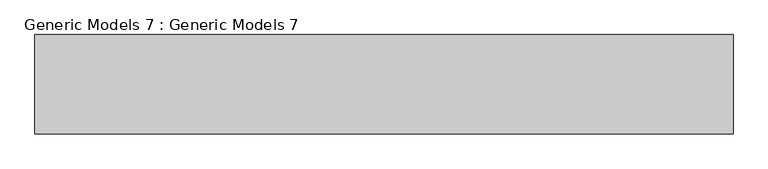
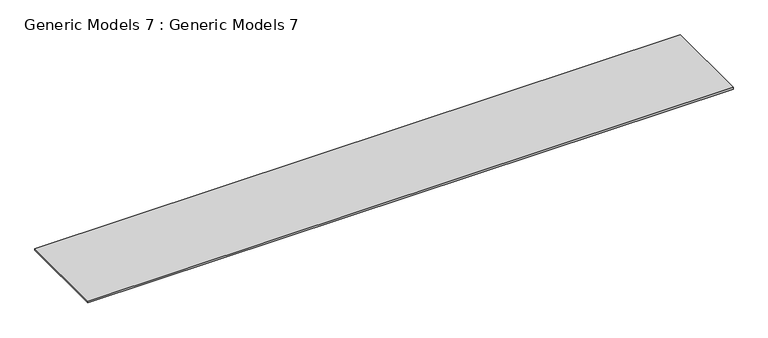
"""IFC4 building model written with IfcOpenShell, lengths in millimetres: proxy geometry, Generic Models 7 : Generic Models 7."""

from ifc_helpers import new_model, si_unit, frame, origin, place, context, project, spatial, polyline, outline, extrude, source, transform, mapped, element, save


def generic_models_7_generic_models_7_b80b7fbc(model_context):
    return source(origin(), model_context, "Body", "SweptSolid", [
        extrude(outline(polyline([(-22815.74674, -19186.7131479), (33752.7751942, -19186.7131479), (33752.7751942, -27224.2253147), (-22815.74674, -27224.2253147), (-22815.74674, -19186.7131479)])), frame((0.0, 0.0, -152.4), z_axis=(0.0, 0.0, 1.0), x_axis=(1.0, 0.0, 0.0)), (0.0, 0.0, 1.0), 152.4),
    ])


if __name__ == "__main__":
    model = new_model("IFC4")
    model_context = context("Model", 3, world=origin())
    ifc_project = project(units=[si_unit("LENGTHUNIT", "METRE", prefix="MILLI")], contexts=[model_context])
    site = spatial("IfcSite", under=ifc_project)
    building = spatial("IfcBuilding", under=site)
    placement = place(None, origin())
    generic_models_7_generic_models_7_shape = generic_models_7_generic_models_7_b80b7fbc(model_context)
    element("IfcBuildingElementProxy", 1, Name="Generic Models 7 : Generic Models 7", ObjectType="Generic Models 7 : Generic Models 7", at=placement, inside=building, context=model_context, shape_type="MappedRepresentation", body=[
        mapped(generic_models_7_generic_models_7_shape, transform((0.0, 0.0, 0.0), x_axis=(1.0, 0.0, 0.0), y_axis=(0.0, 1.0, 0.0), z_axis=(0.0, 0.0, 1.0))),
    ])
    save(model, "model.ifc")
